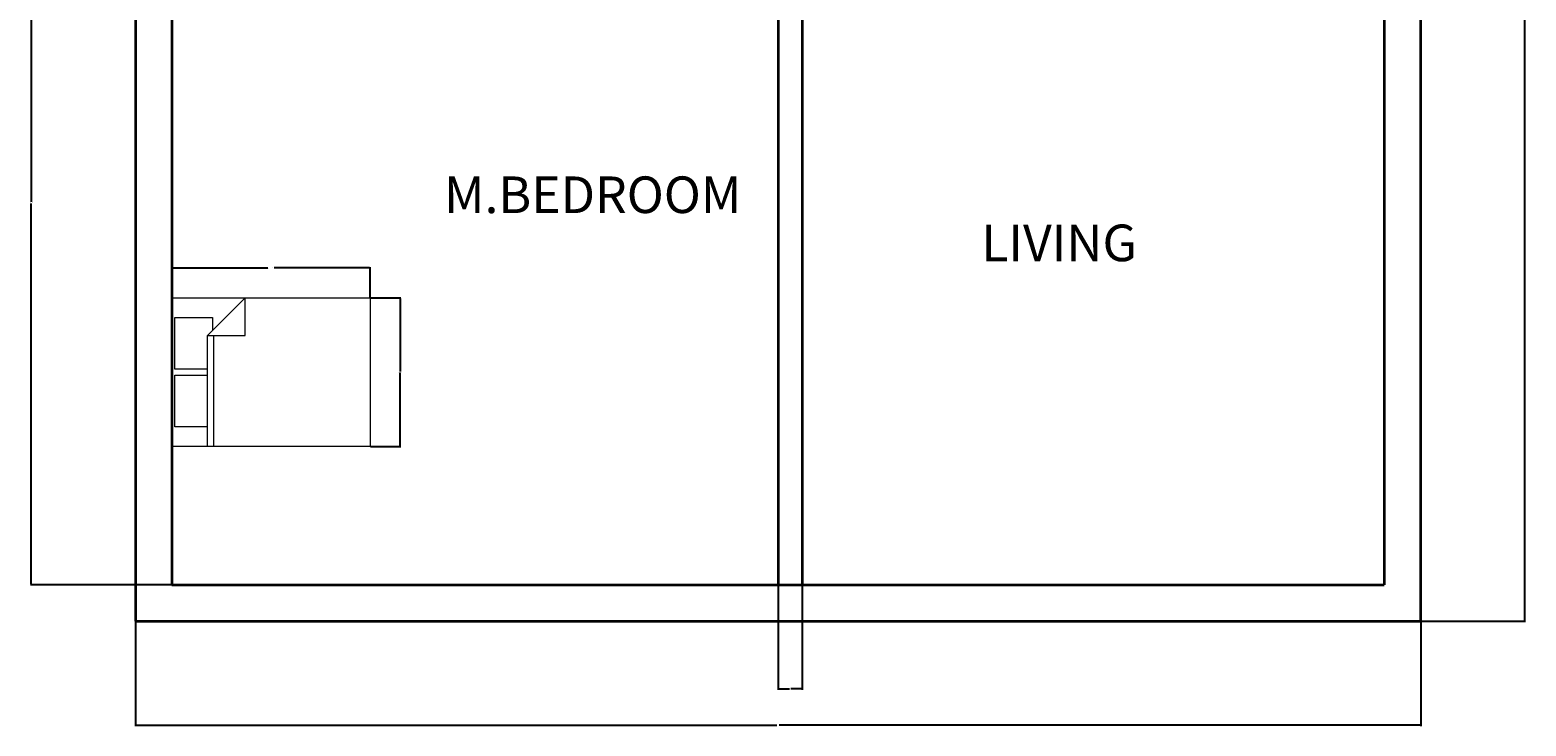
# Model space of a CAD drawing. Units: inches. Extents: x 3024 to 3952, y 1308 to 1863.
# Tile 28 of 29: x 3582 to 3952, y 1308 to 1481. Entities that reach past the tile are written whole.
import ezdxf

# ---------------------------------------------------------------- set-up
doc = ezdxf.new("R2010")
doc.units = ezdxf.units.IN
for name, color, linetype, lineweight in [('A-ANNO-DIMS', 2, 'Continuous', 18), ('A-AREA-IDEN', 7, 'Continuous', 18), ('A-FURN', 8, 'Continuous', 18), ('A-WALL', 7, 'Continuous', 35)]:
    doc.layers.add(name, color=color, linetype=linetype, lineweight=lineweight)
doc.styles.get("Standard").update_dxf_attribs({"font": 'arial.ttf'})
doc.dimstyles.get("Standard").update_dxf_attribs({"dimtxt": 0.18, "dimasz": 0.18, "dimexe": 0.18, "dimexo": 0.0625, "dimgap": 0.09, "dimtad": 0, "dimtih": 1, "dimtoh": 1, "dimdec": 4, "dimzin": 0, "dimdsep": 46, "dimtxsty": 'Standard', "dimcen": 0.09, "dimadec": 0, "dimazin": 0, "dimtfac": 1, "dimtdec": 4, "dimtofl": 0, "dimtmove": 0, "dimatfit": 3, "dimfxl": 1, "dimtolj": 1, "dimtzin": 0, "dimarcsym": 0})

# ---------------------------------------------------------------- blocks, each defined once
blk = doc.blocks.new('Bed - Queen')
for p, q in [((0, -80.00003), (0, 0)), ((0, 0), (59.99999, 0)), ((59.99999, 0), (59.99999, -80.00003)), ((7.99999, -1.2), (28.79998, -1.2)), ((7.99999, -14.4), (7.99999, -1.2)), ((28.79998, -1.2), (28.79998, -14.4)), ((31.19999, -1.2), (51.99999, -1.2)), ((31.19999, -14.4), (31.19999, -1.2)), ((51.99999, -1.2), (51.99999, -16.4)), ((0, -14.4), (44.8, -14.4)), ((44.8, -16.8), (0, -16.8)), ((59.99999, -29.6), (44.8, -14.4)), ((44.8, -14.4), (44.8, -29.6)), ((51.99999, -16.4), (46.79936, -16.4)), ((44.8, -29.6), (59.99999, -29.6)), ((59.99999, -80.00003), (0, -80.00003))]:
    blk.add_line(p, q)
blk = doc.blocks.new('*D18')
at = {"layer": 'A-ANNO-DIMS', "color": 0, "lineweight": -2, "transparency": 16777216}
for p, q in [((3616.64, 1414.52), (3616.64, 1422.01)), ((3616.82, 1421.83), (3640.38, 1421.83)), ((3665.58, 1421.83), (3642.01, 1421.83)), ((3665.76, 1414.52), (3665.76, 1422.01))]:
    blk.add_line(p, q, dxfattribs=at)
at = {"layer": 'A-ANNO-DIMS', "color": 0, "transparency": 16777216}
for points in [[(3616.82, 1421.86), (3616.82, 1421.8), (3616.64, 1421.83)], [(3665.58, 1421.86), (3665.58, 1421.8), (3665.76, 1421.83)]]:
    blk.add_solid(points, dxfattribs=at)
at = {"layer": 'Defpoints', "color": 0, "transparency": 16777216}
for p in [(3616.64, 1421.83), (3616.64, 1414.46), (3665.76, 1414.46)]:
    blk.add_point(p, dxfattribs=at)
at = {"layer": 'A-ANNO-DIMS', "color": 0, "transparency": 16777216, "insert": (3641.2, 1421.83), "char_height": 0.18, "attachment_point": 5}
blk.add_mtext('\\A1;BED 49 TYP.', dxfattribs=at)
blk = doc.blocks.new('*D19')
at = {"layer": 'A-ANNO-DIMS', "color": 0, "lineweight": -2, "transparency": 16777216}
for p, q in [((3665.82, 1414.46), (3673.3, 1414.46)), ((3673.12, 1414.28), (3673.12, 1396.22)), ((3673.12, 1377.8), (3673.12, 1395.86)), ((3665.82, 1377.62), (3673.3, 1377.62))]:
    blk.add_line(p, q, dxfattribs=at)
at = {"layer": 'A-ANNO-DIMS', "color": 0, "transparency": 16777216}
for points in [[(3673.09, 1414.28), (3673.15, 1414.28), (3673.12, 1414.46)], [(3673.09, 1377.8), (3673.15, 1377.8), (3673.12, 1377.62)]]:
    blk.add_solid(points, dxfattribs=at)
at = {"layer": 'Defpoints', "color": 0, "transparency": 16777216}
for p in [(3665.76, 1414.46), (3673.12, 1414.46), (3665.76, 1377.62)]:
    blk.add_point(p, dxfattribs=at)
at = {"layer": 'A-ANNO-DIMS', "color": 0, "transparency": 16777216, "insert": (3673.12, 1396.04), "char_height": 0.18, "attachment_point": 5}
blk.add_mtext('\\A1;37 TYP.', dxfattribs=at)
blk = doc.blocks.new('*D81')
at = {"layer": 'A-ANNO-DIMS', "color": 0, "lineweight": -2, "transparency": 16777216}
for p, q in [((3607.64, 1334.38), (3607.64, 1308.49)), ((3925.64, 1334.38), (3925.64, 1308.49)), ((3607.82, 1308.67), (3766.35, 1308.67)), ((3925.46, 1308.67), (3766.93, 1308.67))]:
    blk.add_line(p, q, dxfattribs=at)
at = {"layer": 'A-ANNO-DIMS', "color": 0, "transparency": 16777216}
for points in [[(3607.82, 1308.7), (3607.82, 1308.64), (3607.64, 1308.67)], [(3925.46, 1308.7), (3925.46, 1308.64), (3925.64, 1308.67)]]:
    blk.add_solid(points, dxfattribs=at)
at = {"layer": 'Defpoints', "color": 0, "transparency": 16777216}
for p in [(3607.64, 1334.44), (3925.64, 1334.44), (3925.64, 1308.67)]:
    blk.add_point(p, dxfattribs=at)
at = {"layer": 'A-ANNO-DIMS', "color": 0, "transparency": 16777216, "insert": (3766.64, 1308.67), "char_height": 0.18, "attachment_point": 5}
blk.add_mtext('\\A1;318', dxfattribs=at)
blk = doc.blocks.new('*D82')
at = {"layer": 'A-ANNO-DIMS', "color": 0, "lineweight": -2, "transparency": 16777216}
for p, q in [((3925.7, 1787.61), (3951.59, 1787.61)), ((3951.41, 1787.43), (3951.41, 1561.21)), ((3951.41, 1334.62), (3951.41, 1560.84)), ((3925.7, 1334.44), (3951.59, 1334.44))]:
    blk.add_line(p, q, dxfattribs=at)
at = {"layer": 'A-ANNO-DIMS', "color": 0, "transparency": 16777216}
for points in [[(3951.38, 1787.43), (3951.44, 1787.43), (3951.41, 1787.61)], [(3951.38, 1334.62), (3951.44, 1334.62), (3951.41, 1334.44)]]:
    blk.add_solid(points, dxfattribs=at)
at = {"layer": 'Defpoints', "color": 0, "transparency": 16777216}
for p in [(3925.64, 1787.61), (3951.41, 1787.61), (3925.64, 1334.44)]:
    blk.add_point(p, dxfattribs=at)
at = {"layer": 'A-ANNO-DIMS', "color": 0, "transparency": 16777216, "insert": (3951.41, 1561.02), "char_height": 0.18, "attachment_point": 5}
blk.add_mtext('\\A1;453.2', dxfattribs=at)
blk = doc.blocks.new('*D93')
at = {"layer": 'A-ANNO-DIMS', "color": 0, "lineweight": -2, "transparency": 16777216}
for p, q in [((3616.64, 1343.5), (3616.64, 1813.56)), ((3616.82, 1813.38), (3691.36, 1813.38)), ((3766.46, 1813.38), (3691.92, 1813.38)), ((3766.64, 1343.5), (3766.64, 1813.56))]:
    blk.add_line(p, q, dxfattribs=at)
at = {"layer": 'A-ANNO-DIMS', "color": 0, "transparency": 16777216}
for points in [[(3616.82, 1813.41), (3616.82, 1813.35), (3616.64, 1813.38)], [(3766.46, 1813.41), (3766.46, 1813.35), (3766.64, 1813.38)]]:
    blk.add_solid(points, dxfattribs=at)
at = {"layer": 'Defpoints', "color": 0, "transparency": 16777216}
for p in [(3766.64, 1813.38), (3616.64, 1343.44), (3766.64, 1343.44)]:
    blk.add_point(p, dxfattribs=at)
at = {"layer": 'A-ANNO-DIMS', "color": 0, "transparency": 16777216, "insert": (3691.64, 1813.38), "char_height": 0.18, "attachment_point": 5}
blk.add_mtext('\\A1;150', dxfattribs=at)
blk = doc.blocks.new('*D97')
at = {"layer": 'A-ANNO-DIMS', "color": 0, "lineweight": -2, "transparency": 16777216}
for p, q in [((3616.58, 1532.52), (3581.68, 1532.52)), ((3581.86, 1532.34), (3581.86, 1438.16)), ((3581.86, 1343.62), (3581.86, 1437.8)), ((3616.58, 1343.44), (3581.68, 1343.44))]:
    blk.add_line(p, q, dxfattribs=at)
at = {"layer": 'A-ANNO-DIMS', "color": 0, "transparency": 16777216}
for points in [[(3581.83, 1532.34), (3581.89, 1532.34), (3581.86, 1532.52)], [(3581.83, 1343.62), (3581.89, 1343.62), (3581.86, 1343.44)]]:
    blk.add_solid(points, dxfattribs=at)
at = {"layer": 'Defpoints', "color": 0, "transparency": 16777216}
for p in [(3581.86, 1532.52), (3616.64, 1532.52), (3616.64, 1343.44)]:
    blk.add_point(p, dxfattribs=at)
at = {"layer": 'A-ANNO-DIMS', "color": 0, "transparency": 16777216, "insert": (3581.86, 1437.98), "char_height": 0.18, "attachment_point": 5}
blk.add_mtext('\\A1;189.1', dxfattribs=at)
blk = doc.blocks.new('*D102')
at = {"layer": 'A-ANNO-DIMS', "color": 0, "lineweight": -2, "transparency": 16777216}
for p, q in [((3766.64, 1343.38), (3766.64, 1317.49)), ((3772.64, 1343.38), (3772.64, 1317.49)), ((3766.82, 1317.67), (3769.49, 1317.67)), ((3772.46, 1317.67), (3769.79, 1317.67))]:
    blk.add_line(p, q, dxfattribs=at)
at = {"layer": 'A-ANNO-DIMS', "color": 0, "transparency": 16777216}
for points in [[(3766.82, 1317.7), (3766.82, 1317.64), (3766.64, 1317.67)], [(3772.46, 1317.7), (3772.46, 1317.64), (3772.64, 1317.67)]]:
    blk.add_solid(points, dxfattribs=at)
at = {"layer": 'Defpoints', "color": 0, "transparency": 16777216}
for p in [(3766.64, 1343.44), (3772.64, 1343.44), (3766.64, 1317.67)]:
    blk.add_point(p, dxfattribs=at)
at = {"layer": 'A-ANNO-DIMS', "color": 0, "transparency": 16777216, "insert": (3769.64, 1317.67), "char_height": 0.18, "attachment_point": 5}
blk.add_mtext('\\A1;6', dxfattribs=at)

msp = doc.modelspace()

# ---------------------------------------------------------------- linework, layer by layer
at = {"layer": 'A-WALL'}
for p, q in [((3607.6376, 1787.6064), (3607.6376, 1334.4405)), ((3925.6376, 1787.6064), (3925.6376, 1334.4405)), ((3616.6376, 1688.6064), (3616.6376, 1343.4405)), ((3772.6376, 1500.4537), (3772.6376, 1343.4405)), ((3916.6376, 1501.5221), (3916.6376, 1343.4405)), ((3766.6376, 1494.4537), (3766.6376, 1343.4405)), ((3616.6376, 1343.4405), (3916.6376, 1343.4405)), ((3607.6376, 1334.4405), (3925.6376, 1334.4405))]:
    msp.add_line(p, q, dxfattribs=at)

# ---------------------------------------------------------------- block references
at = {"layer": 'A-FURN', "xscale": 0.613989453470478, "yscale": 0.613989453470478, "zscale": 0.613989453470478, "rotation": 89.9999999999993}
msp.add_blockref('Bed - Queen', (3616.6376, 1377.6193), dxfattribs=at)

# ---------------------------------------------------------------- texts
at = {"layer": 'A-AREA-IDEN'}
for s, p in [('M.BEDROOM', (3683.9978, 1435.4125)), ('LIVING', (3816.9314, 1423.5052))]:
    msp.add_text(s, height=9.05874, dxfattribs=at).set_placement(p)

# ---------------------------------------------------------------- dimensions: what is measured, and where the dimension line sits
at = {"layer": 'A-ANNO-DIMS'}
for base, p1, p2, picture, middle in [((3766.6376, 1813.3814), (3616.6376, 1343.4405), (3766.6376, 1343.4405), '*D93', (3691.6376, 1813.3814)), ((3925.6376, 1308.6655), (3607.6376, 1334.4405), (3925.6376, 1334.4405), '*D81', (3766.6376, 1308.6655))]:
    dim = msp.add_linear_dim(base=base, p1=p1, p2=p2, dimstyle='Standard', override={"dimdec": 0, "dimlfac": 1, "dimrnd": 0, "dimzin": 0, "dimdsep": 46, "dimlunit": 2}, dxfattribs=at)
    dim.commit()
    dim.dimension.update_dxf_attribs({"geometry": picture, "text_midpoint": middle})
for base, p1, p2, angle, override, picture, middle in [((3951.4126, 1787.6064), (3925.6376, 1334.4405), (3925.6376, 1787.6064), 90, {"dimdec": 1, "dimlfac": 1, "dimrnd": 0, "dimzin": 0, "dimdsep": 46, "dimlunit": 2}, '*D82', (3951.4126, 1561.0234)), ((3581.8626, 1532.5223), (3616.6376, 1343.4405), (3616.6376, 1532.5223), 90, {"dimdec": 1, "dimlfac": 1, "dimrnd": 0, "dimzin": 0, "dimdsep": 46, "dimlunit": 2}, '*D97', (3581.8626, 1437.9814)), ((3766.6376, 1317.6655), (3772.6376, 1343.4405), (3766.6376, 1343.4405), 180, {"dimdec": 0, "dimlfac": 1, "dimrnd": 0, "dimzin": 0, "dimdsep": 46, "dimlunit": 2}, '*D102', (3769.6376, 1317.6655))]:
    dim = msp.add_linear_dim(base=base, p1=p1, p2=p2, angle=angle, dimstyle='Standard', override=override, dxfattribs=at)
    dim.commit()
    dim.dimension.update_dxf_attribs({"geometry": picture, "text_midpoint": middle})
for base, p1, p2, angle, text, picture, middle in [((3616.6376, 1421.8265), (3665.7568, 1414.4587), (3616.6376, 1414.4587), 180, 'BED <> TYP.', '*D18', (3641.1972, 1421.8265)), ((3673.1246, 1414.4587), (3665.7568, 1377.6193), (3665.7568, 1414.4587), 90, '<> TYP.', '*D19', (3673.1246, 1396.039))]:
    dim = msp.add_linear_dim(base=base, p1=p1, p2=p2, angle=angle, text=text, dimstyle='Standard', override={"dimdec": 0, "dimlfac": 1, "dimrnd": 0, "dimzin": 0, "dimdsep": 46, "dimlunit": 2}, dxfattribs=at)
    dim.commit()
    dim.dimension.update_dxf_attribs({"geometry": picture, "text_midpoint": middle})

doc.saveas('drawing.dxf')
